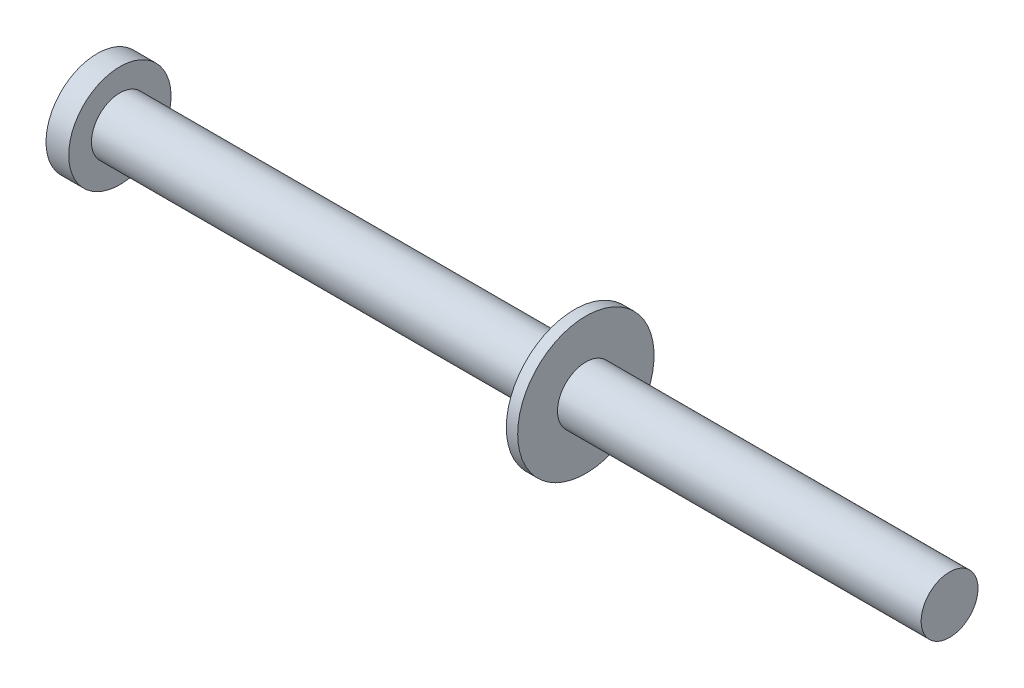
ISO-10303-21;
HEADER;
FILE_DESCRIPTION(('STEP AP214'),'2;1');
FILE_NAME('part.step','',(''),(''),'','','');
FILE_SCHEMA(('AUTOMOTIVE_DESIGN { 1 0 10303 214 1 1 1 1 }'));
ENDSEC;
DATA;
#1=APPLICATION_CONTEXT('core data for automotive mechanical design processes');
#2=APPLICATION_PROTOCOL_DEFINITION('international standard','automotive_design',2000,#1);
#3=PRODUCT_CONTEXT('',#1,'mechanical');
#4=PRODUCT('Part','Part','',(#3));
#5=PRODUCT_RELATED_PRODUCT_CATEGORY('part','',(#4));
#6=PRODUCT_DEFINITION_FORMATION('','',#4);
#7=PRODUCT_DEFINITION_CONTEXT('part definition',#1,'design');
#8=PRODUCT_DEFINITION('design','',#6,#7);
#9=PRODUCT_DEFINITION_SHAPE('','',#8);
#10=(LENGTH_UNIT() NAMED_UNIT(*) SI_UNIT(.MILLI.,.METRE.));
#11=(NAMED_UNIT(*) PLANE_ANGLE_UNIT() SI_UNIT($,.RADIAN.));
#12=(NAMED_UNIT(*) SI_UNIT($,.STERADIAN.) SOLID_ANGLE_UNIT());
#13=UNCERTAINTY_MEASURE_WITH_UNIT(LENGTH_MEASURE(1.E-05),#10,'distance_accuracy_value','');
#14=(GEOMETRIC_REPRESENTATION_CONTEXT(3) GLOBAL_UNCERTAINTY_ASSIGNED_CONTEXT((#13)) GLOBAL_UNIT_ASSIGNED_CONTEXT((#10,
#11,#12)) REPRESENTATION_CONTEXT('',''));
#15=CARTESIAN_POINT('',(0.,0.,0.));
#16=DIRECTION('',(0.,0.,1.));
#17=DIRECTION('',(1.,0.,0.));
#18=AXIS2_PLACEMENT_3D('',#15,#16,#17);
#19=CARTESIAN_POINT('',(64.,0.,0.));
#20=DIRECTION('',(-1.,0.,0.));
#21=DIRECTION('',(0.,0.,1.));
#22=AXIS2_PLACEMENT_3D('',#19,#20,#21);
#23=CYLINDRICAL_SURFACE('',#22,5.);
#24=CARTESIAN_POINT('',(64.,0.,0.));
#25=DIRECTION('',(1.,0.,0.));
#26=DIRECTION('',(0.,0.,-1.));
#27=AXIS2_PLACEMENT_3D('',#24,#25,#26);
#28=CIRCLE('',#27,5.);
#29=CARTESIAN_POINT('',(64.,0.,-5.));
#30=VERTEX_POINT('',#29);
#31=EDGE_CURVE('E46',#30,#30,#28,.T.);
#32=ORIENTED_EDGE('',*,*,#31,.F.);
#33=EDGE_LOOP('',(#32));
#34=FACE_BOUND('',#33,.T.);
#35=CARTESIAN_POINT('',(0.,0.,0.));
#36=DIRECTION('',(1.,0.,0.));
#37=DIRECTION('',(0.,0.,-1.));
#38=AXIS2_PLACEMENT_3D('',#35,#36,#37);
#39=CIRCLE('',#38,5.);
#40=CARTESIAN_POINT('',(0.,0.,-5.));
#41=VERTEX_POINT('',#40);
#42=EDGE_CURVE('E45',#41,#41,#39,.T.);
#43=ORIENTED_EDGE('',*,*,#42,.T.);
#44=EDGE_LOOP('',(#43));
#45=FACE_BOUND('',#44,.T.);
#46=ADVANCED_FACE('F39',(#34,#45),#23,.T.);
#47=CARTESIAN_POINT('',(64.,0.,0.));
#48=DIRECTION('',(1.,0.,0.));
#49=DIRECTION('',(0.,0.,-1.));
#50=AXIS2_PLACEMENT_3D('',#47,#48,#49);
#51=PLANE('',#50);
#52=ORIENTED_EDGE('',*,*,#31,.T.);
#53=EDGE_LOOP('',(#52));
#54=FACE_BOUND('',#53,.T.);
#55=ADVANCED_FACE('F88',(#54),#51,.T.);
#56=CARTESIAN_POINT('',(-2.,0.,0.));
#57=DIRECTION('',(1.,0.,0.));
#58=DIRECTION('',(0.,0.,-1.));
#59=AXIS2_PLACEMENT_3D('',#56,#57,#58);
#60=CYLINDRICAL_SURFACE('',#59,12.);
#61=CARTESIAN_POINT('',(-2.,0.,0.));
#62=DIRECTION('',(-1.,0.,0.));
#63=DIRECTION('',(0.,0.,1.));
#64=AXIS2_PLACEMENT_3D('',#61,#62,#63);
#65=CIRCLE('',#64,12.);
#66=CARTESIAN_POINT('',(-2.,0.,12.));
#67=VERTEX_POINT('',#66);
#68=EDGE_CURVE('E54',#67,#67,#65,.T.);
#69=ORIENTED_EDGE('',*,*,#68,.F.);
#70=EDGE_LOOP('',(#69));
#71=FACE_BOUND('',#70,.T.);
#72=CARTESIAN_POINT('',(0.,0.,0.));
#73=DIRECTION('',(-1.,0.,0.));
#74=DIRECTION('',(0.,0.,1.));
#75=AXIS2_PLACEMENT_3D('',#72,#73,#74);
#76=CIRCLE('',#75,12.);
#77=CARTESIAN_POINT('',(0.,0.,12.));
#78=VERTEX_POINT('',#77);
#79=EDGE_CURVE('E59',#78,#78,#76,.T.);
#80=ORIENTED_EDGE('',*,*,#79,.T.);
#81=EDGE_LOOP('',(#80));
#82=FACE_BOUND('',#81,.T.);
#83=ADVANCED_FACE('F93',(#71,#82),#60,.T.);
#84=CARTESIAN_POINT('',(-2.,0.,0.));
#85=DIRECTION('',(-1.,0.,0.));
#86=DIRECTION('',(0.,0.,1.));
#87=AXIS2_PLACEMENT_3D('',#84,#85,#86);
#88=PLANE('',#87);
#89=CARTESIAN_POINT('',(-2.,0.,0.));
#90=DIRECTION('',(-1.,0.,0.));
#91=DIRECTION('',(0.,0.,1.));
#92=AXIS2_PLACEMENT_3D('',#89,#90,#91);
#93=CIRCLE('',#92,5.);
#94=CARTESIAN_POINT('',(-2.,0.,5.));
#95=VERTEX_POINT('',#94);
#96=EDGE_CURVE('E10',#95,#95,#93,.T.);
#97=ORIENTED_EDGE('',*,*,#96,.F.);
#98=EDGE_LOOP('',(#97));
#99=FACE_BOUND('',#98,.T.);
#100=ORIENTED_EDGE('',*,*,#68,.T.);
#101=EDGE_LOOP('',(#100));
#102=FACE_BOUND('',#101,.T.);
#103=ADVANCED_FACE('F105',(#99,#102),#88,.T.);
#104=CARTESIAN_POINT('',(0.,0.,0.));
#105=DIRECTION('',(-1.,0.,0.));
#106=DIRECTION('',(0.,0.,1.));
#107=AXIS2_PLACEMENT_3D('',#104,#105,#106);
#108=PLANE('',#107);
#109=ORIENTED_EDGE('',*,*,#42,.F.);
#110=EDGE_LOOP('',(#109));
#111=FACE_BOUND('',#110,.T.);
#112=ORIENTED_EDGE('',*,*,#79,.F.);
#113=EDGE_LOOP('',(#112));
#114=FACE_BOUND('',#113,.T.);
#115=ADVANCED_FACE('F98',(#111,#114),#108,.F.);
#116=CARTESIAN_POINT('',(-82.,0.,0.));
#117=DIRECTION('',(1.,0.,0.));
#118=DIRECTION('',(0.,0.,-1.));
#119=AXIS2_PLACEMENT_3D('',#116,#117,#118);
#120=CYLINDRICAL_SURFACE('',#119,5.);
#121=CARTESIAN_POINT('',(-82.,0.,0.));
#122=DIRECTION('',(-1.,0.,0.));
#123=DIRECTION('',(0.,0.,1.));
#124=AXIS2_PLACEMENT_3D('',#121,#122,#123);
#125=CIRCLE('',#124,5.);
#126=CARTESIAN_POINT('',(-82.,0.,5.));
#127=VERTEX_POINT('',#126);
#128=EDGE_CURVE('E52',#127,#127,#125,.T.);
#129=ORIENTED_EDGE('',*,*,#128,.F.);
#130=EDGE_LOOP('',(#129));
#131=FACE_BOUND('',#130,.T.);
#132=ORIENTED_EDGE('',*,*,#96,.T.);
#133=EDGE_LOOP('',(#132));
#134=FACE_BOUND('',#133,.T.);
#135=ADVANCED_FACE('F101',(#131,#134),#120,.T.);
#136=CARTESIAN_POINT('',(-86.,0.,0.));
#137=DIRECTION('',(1.,0.,0.));
#138=DIRECTION('',(0.,0.,-1.));
#139=AXIS2_PLACEMENT_3D('',#136,#137,#138);
#140=CYLINDRICAL_SURFACE('',#139,9.);
#141=CARTESIAN_POINT('',(-86.,0.,0.));
#142=DIRECTION('',(-1.,0.,0.));
#143=DIRECTION('',(0.,0.,1.));
#144=AXIS2_PLACEMENT_3D('',#141,#142,#143);
#145=CIRCLE('',#144,9.);
#146=CARTESIAN_POINT('',(-86.,0.,9.));
#147=VERTEX_POINT('',#146);
#148=EDGE_CURVE('E62',#147,#147,#145,.T.);
#149=ORIENTED_EDGE('',*,*,#148,.F.);
#150=EDGE_LOOP('',(#149));
#151=FACE_BOUND('',#150,.T.);
#152=CARTESIAN_POINT('',(-82.,0.,0.));
#153=DIRECTION('',(-1.,0.,0.));
#154=DIRECTION('',(0.,0.,1.));
#155=AXIS2_PLACEMENT_3D('',#152,#153,#154);
#156=CIRCLE('',#155,9.);
#157=CARTESIAN_POINT('',(-82.,0.,9.));
#158=VERTEX_POINT('',#157);
#159=EDGE_CURVE('E66',#158,#158,#156,.T.);
#160=ORIENTED_EDGE('',*,*,#159,.T.);
#161=EDGE_LOOP('',(#160));
#162=FACE_BOUND('',#161,.T.);
#163=ADVANCED_FACE('F74',(#151,#162),#140,.T.);
#164=CARTESIAN_POINT('',(-86.,0.,0.));
#165=DIRECTION('',(-1.,0.,0.));
#166=DIRECTION('',(0.,0.,1.));
#167=AXIS2_PLACEMENT_3D('',#164,#165,#166);
#168=PLANE('',#167);
#169=ORIENTED_EDGE('',*,*,#148,.T.);
#170=EDGE_LOOP('',(#169));
#171=FACE_BOUND('',#170,.T.);
#172=ADVANCED_FACE('F77',(#171),#168,.T.);
#173=CARTESIAN_POINT('',(-82.,0.,0.));
#174=DIRECTION('',(-1.,0.,0.));
#175=DIRECTION('',(0.,0.,1.));
#176=AXIS2_PLACEMENT_3D('',#173,#174,#175);
#177=PLANE('',#176);
#178=ORIENTED_EDGE('',*,*,#128,.T.);
#179=EDGE_LOOP('',(#178));
#180=FACE_BOUND('',#179,.T.);
#181=ORIENTED_EDGE('',*,*,#159,.F.);
#182=EDGE_LOOP('',(#181));
#183=FACE_BOUND('',#182,.T.);
#184=ADVANCED_FACE('F78',(#180,#183),#177,.F.);
#185=CLOSED_SHELL('',(#46,#55,#83,#103,#115,#135,#163,#172,#184));
#186=MANIFOLD_SOLID_BREP('B2',#185);
#187=ADVANCED_BREP_SHAPE_REPRESENTATION('',(#18,#186),#14);
#188=SHAPE_DEFINITION_REPRESENTATION(#9,#187);
ENDSEC;
END-ISO-10303-21;
